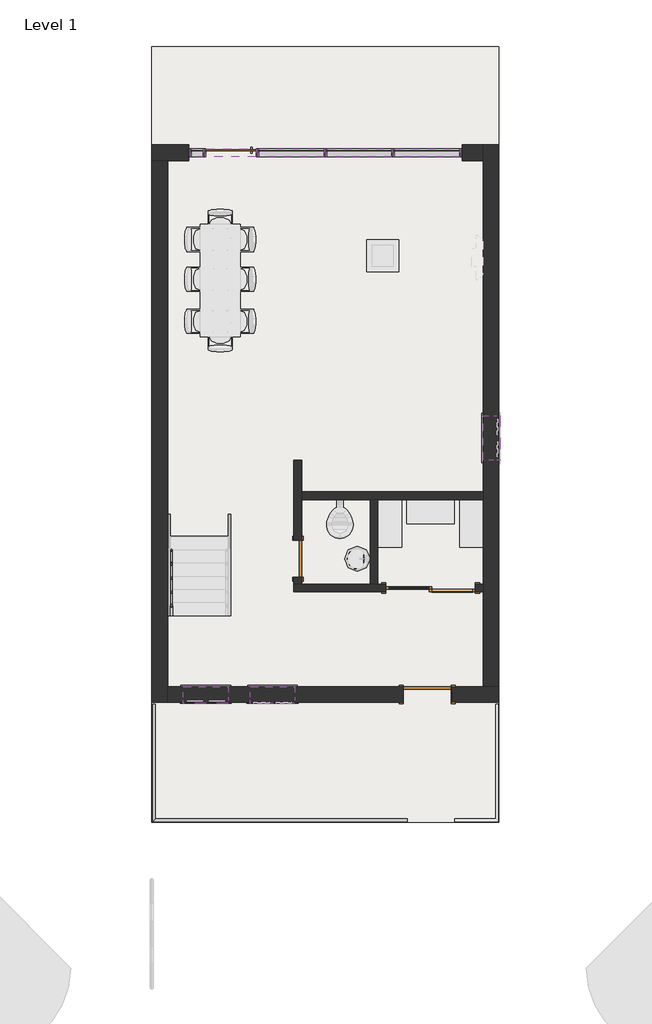
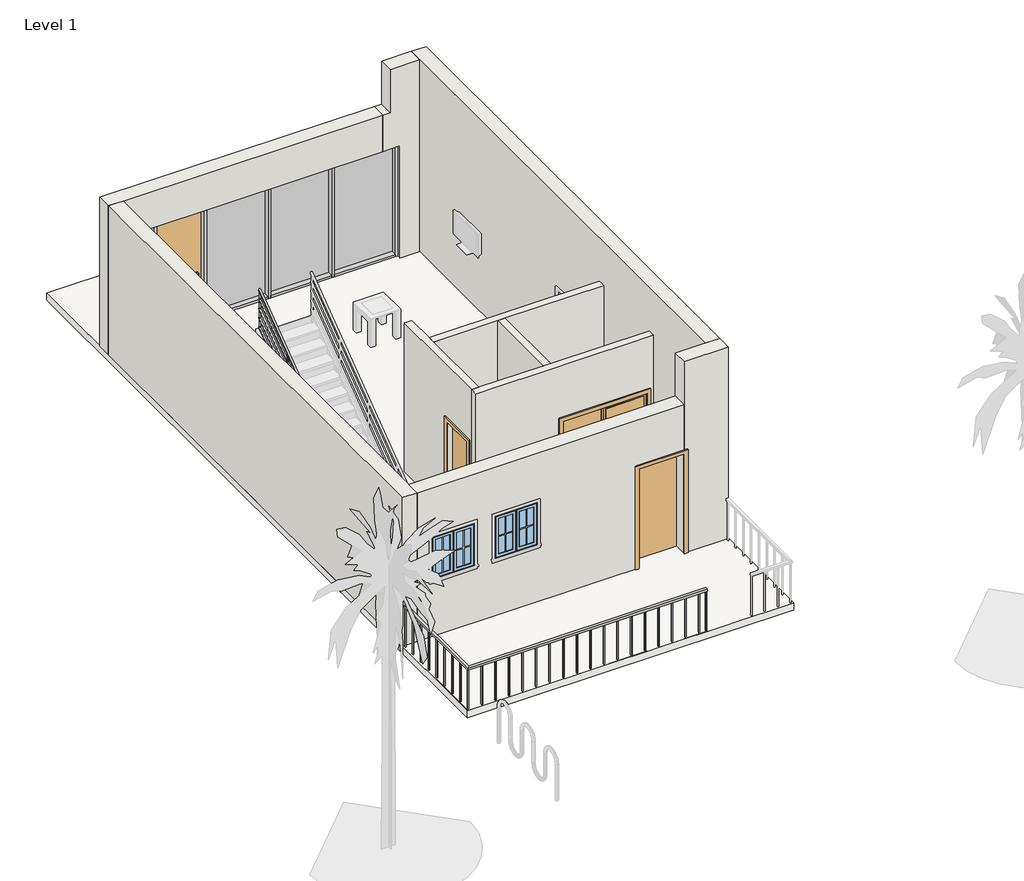
# One storey, part 1 of 2: 15 members, 10 walls, 4 doors, 4 plates, 3 windows, 2 railings, 1 slab.
# Revit data of these elements (continued)
# Materials (continued)
#   "Aluminium": class "Metal", colour RGB 247 247 247, transparency 0, Description = "Aluminium 6061", Cost = 0
#   "Default New Material(6)": class "Generic", colour RGB 191 25 25, transparency 0.9, Cost = 0
#   "Default New Material": class "Generic", colour RGB 211 206 0, transparency 0.8, Cost = 0
#   "Textile - Black": class "Fabric", colour RGB 0 0 0, transparency 0
#   "Ceiling Tile 600 x 600": class "Generic", colour RGB 235 235 235, transparency 0, Description = "Acoustic ceiling tile", Cost = 0
#   "Default Wall": colour RGB 128 128 128, transparency 0, Cost = 0
#   "Default New Material(7)": class "Generic", colour RGB 69 80 94, transparency 0, Cost = 0
#   "Default New Material(9)": class "Generic", colour RGB 63 63 64, transparency 0, Cost = 0
